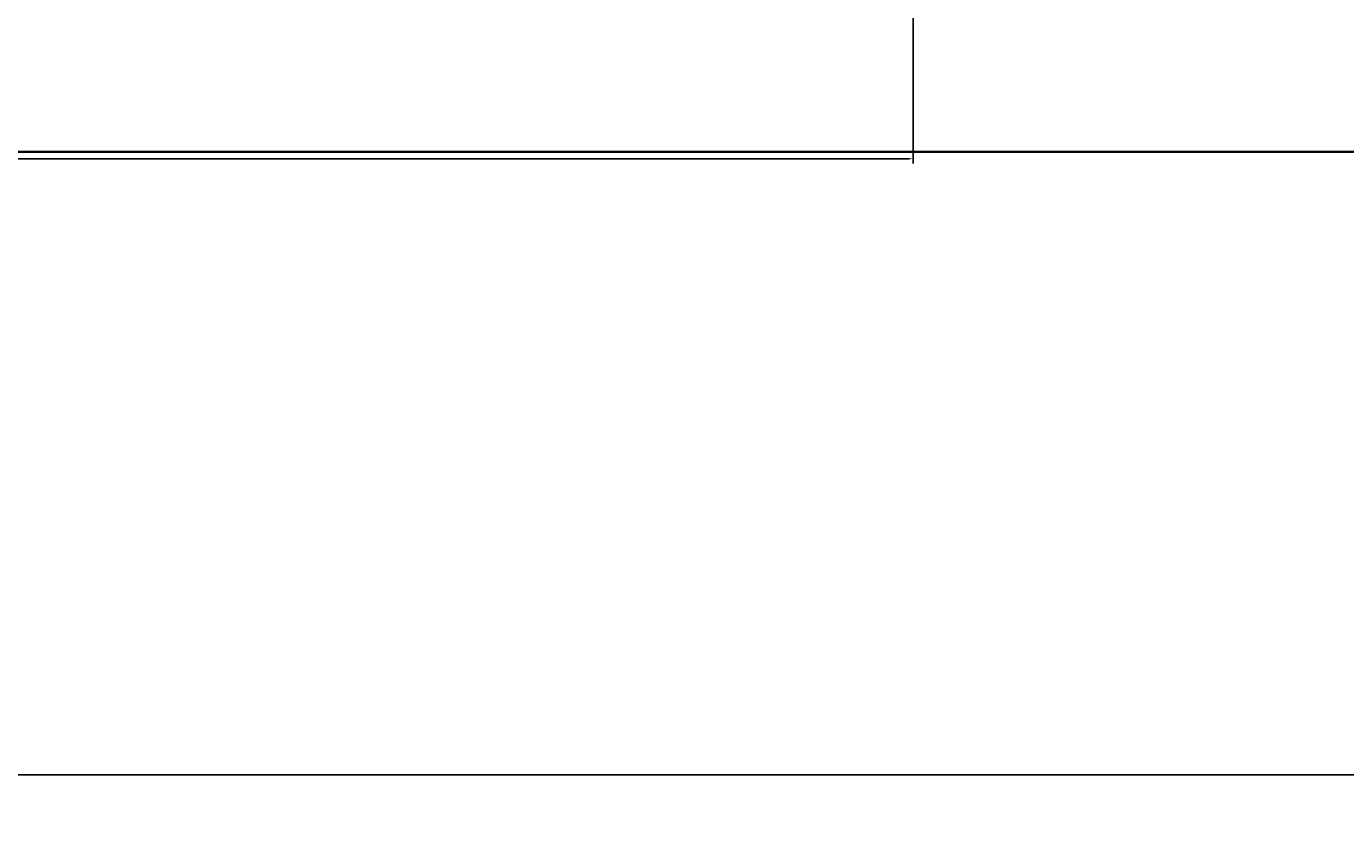
# Model space of a CAD drawing. Units: inches. Extents: x -61 to 1599, y -1316 to 257.
# Tile 6 of 204: x 149 to 200, y -1242 to -1211. Entities that reach past the tile are written whole.
import ezdxf

# ---------------------------------------------------------------- set-up
doc = ezdxf.new("R2010")
doc.units = ezdxf.units.IN
doc.header["$MEASUREMENT"] = 0
doc.layers.add('A-ANNO-DIMS', color=2, linetype='Continuous', lineweight=18)
doc.layers.add('WALLS', color=4, linetype='Continuous', lineweight=35)
doc.styles.get("Standard").update_dxf_attribs({"font": 'arial.ttf'})
doc.dimstyles.get("Standard").update_dxf_attribs({"dimtxt": 0.18, "dimasz": 0.18, "dimexe": 0.18, "dimexo": 0.0625, "dimgap": 0.09, "dimtad": 0, "dimtih": 1, "dimtoh": 1, "dimdec": 0, "dimzin": 0, "dimdsep": 46, "dimlunit": 3, "dimtxsty": 'Standard', "dimcen": 0.09, "dimadec": 0, "dimazin": 0, "dimtfac": 1, "dimtdec": 0, "dimtofl": 0, "dimtmove": 0, "dimatfit": 3, "dimfxl": 1, "dimtolj": 1, "dimtzin": 0, "dimarcsym": 0})

# ---------------------------------------------------------------- blocks, each defined once
blk = doc.blocks.new('*D635')
at = {"layer": 'A-ANNO-DIMS', "color": 0, "lineweight": -2, "transparency": 16777216}
for p, q in [((111.872, -1202.381), (111.872, -1216.391)), ((183.57, -1202.381), (183.57, -1216.391)), ((112.052, -1216.211), (147.193, -1216.211)), ((183.39, -1216.211), (148.248, -1216.211))]:
    blk.add_line(p, q, dxfattribs=at)
at = {"layer": 'A-ANNO-DIMS', "color": 0, "transparency": 16777216}
for points in [[(112.052, -1216.181), (112.052, -1216.241), (111.872, -1216.211)], [(183.39, -1216.181), (183.39, -1216.241), (183.57, -1216.211)]]:
    blk.add_solid(points, dxfattribs=at)
at = {"layer": 'DEFPOINTS', "color": 0, "transparency": 16777216}
for p in [(111.872, -1202.318), (183.57, -1202.318), (183.57, -1216.211)]:
    blk.add_point(p, dxfattribs=at)
at = {"layer": 'A-ANNO-DIMS', "color": 0, "transparency": 16777216, "insert": (147.721, -1216.211), "char_height": 0.18, "attachment_point": 5}
blk.add_mtext('\\A1;72 TYP.', dxfattribs=at)
blk = doc.blocks.new('*D687')
at = {"layer": 'A-ANNO-DIMS', "color": 0, "lineweight": -2, "transparency": 16777216}
for p, q in [((289.418, 181.677), (-61.077, 181.677)), ((-60.897, 181.497), (-60.897, -528.952)), ((-60.897, -1239.765), (-60.897, -529.316)), ((319.64, -1239.945), (-61.077, -1239.945))]:
    blk.add_line(p, q, dxfattribs=at)
at = {"layer": 'A-ANNO-DIMS', "color": 0, "transparency": 16777216}
for points in [[(-60.927, 181.497), (-60.867, 181.497), (-60.897, 181.677)], [(-60.927, -1239.765), (-60.867, -1239.765), (-60.897, -1239.945)]]:
    blk.add_solid(points, dxfattribs=at)
at = {"layer": 'DEFPOINTS', "color": 0, "transparency": 16777216}
for p in [(289.481, 181.677), (-60.897, -1239.945), (319.703, -1239.945)]:
    blk.add_point(p, dxfattribs=at)
at = {"layer": 'A-ANNO-DIMS', "color": 0, "transparency": 16777216, "insert": (-60.897, -529.134), "char_height": 0.18, "attachment_point": 5}
blk.add_mtext('\\A1;1421.6', dxfattribs=at)
blk = doc.blocks.new('*D688')
at = {"layer": 'A-ANNO-DIMS', "color": 0, "lineweight": -2, "transparency": 16777216}
for p, q in [((14.703, -1216.007), (14.703, -1315.725)), ((544.703, -1216.007), (544.703, -1315.725)), ((14.883, -1315.545), (279.414, -1315.545)), ((544.523, -1315.545), (279.991, -1315.545))]:
    blk.add_line(p, q, dxfattribs=at)
at = {"layer": 'A-ANNO-DIMS', "color": 0, "transparency": 16777216}
for points in [[(14.883, -1315.515), (14.883, -1315.575), (14.703, -1315.545)], [(544.523, -1315.515), (544.523, -1315.575), (544.703, -1315.545)]]:
    blk.add_solid(points, dxfattribs=at)
at = {"layer": 'DEFPOINTS', "color": 0, "transparency": 16777216}
for p in [(14.703, -1215.945), (544.703, -1215.945), (544.703, -1315.545)]:
    blk.add_point(p, dxfattribs=at)
at = {"layer": 'A-ANNO-DIMS', "color": 0, "transparency": 16777216, "insert": (279.703, -1315.545), "char_height": 0.18, "attachment_point": 5}
blk.add_mtext('\\A1;530', dxfattribs=at)

msp = doc.modelspace()

# ---------------------------------------------------------------- linework, layer by layer
at = {"layer": 'WALLS'}
msp.add_line((14.7028, -1215.9446), (237.7028, -1215.9446), dxfattribs=at)

# ---------------------------------------------------------------- dimensions: what is measured, and where the dimension line sits
at = {"layer": 'A-ANNO-DIMS'}
dim = msp.add_linear_dim(base=(-60.8972, -1239.9446), p1=(289.4807, 181.6771), p2=(319.7028, -1239.9446), angle=90, dimstyle='Standard', override={"dimdec": 1, "dimlfac": 1, "dimrnd": 0, "dimzin": 0, "dimdsep": 46, "dimlunit": 2}, dxfattribs=at)
dim.commit()
dim.dimension.update_dxf_attribs({"geometry": '*D687', "text_midpoint": (-60.8972, -529.1337)})
dim = msp.add_linear_dim(base=(183.5695, -1216.2111), p1=(111.8719, -1202.3182), p2=(183.5695, -1202.3182), text='<> TYP.', dimstyle='Standard', override={"dimdec": 0, "dimlfac": 1, "dimrnd": 0, "dimzin": 0, "dimdsep": 46, "dimlunit": 2}, dxfattribs=at)
dim.commit()
dim.dimension.update_dxf_attribs({"geometry": '*D635', "text_midpoint": (147.7207, -1216.2111)})
dim = msp.add_linear_dim(base=(544.7028, -1315.5446), p1=(14.7028, -1215.9446), p2=(544.7028, -1215.9446), dimstyle='Standard', override={"dimdec": 0, "dimlfac": 1, "dimrnd": 0, "dimzin": 0, "dimdsep": 46, "dimlunit": 2}, dxfattribs=at)
dim.commit()
dim.dimension.update_dxf_attribs({"geometry": '*D688', "text_midpoint": (279.7028, -1315.5446)})

doc.saveas('drawing.dxf')
